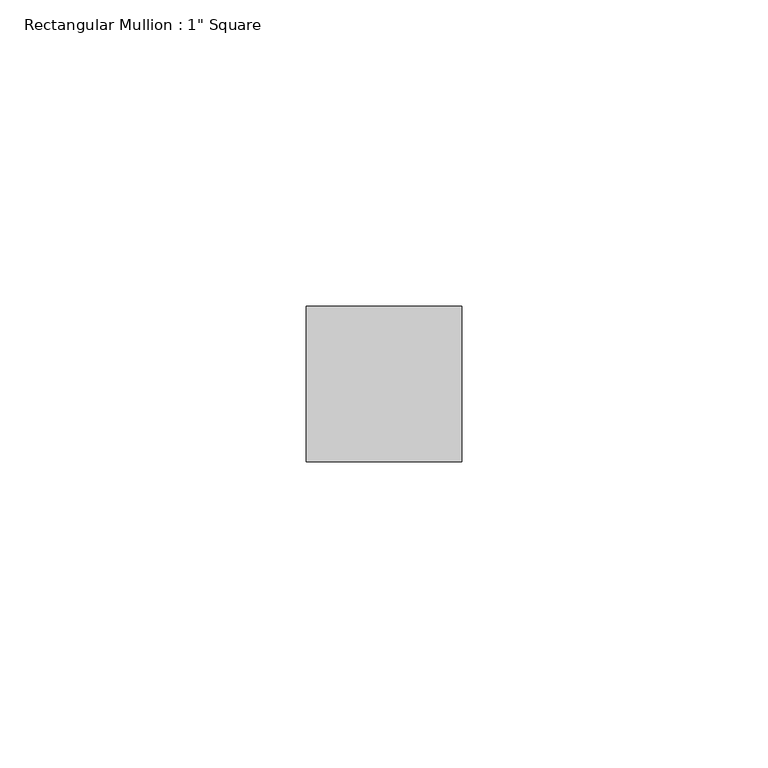
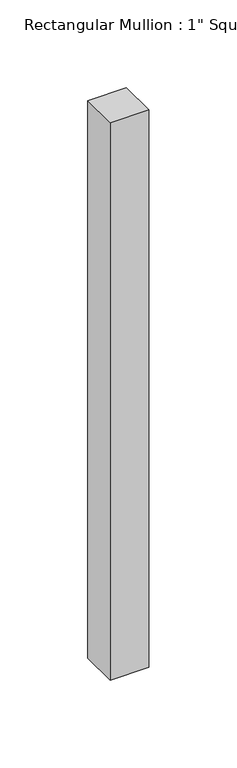
"""IFC4 building model written with IfcOpenShell, lengths in millimetres: member geometry."""

from ifc_helpers import new_model, si_unit, frame, origin, place, context, project, spatial, polyline, outline, extrude, source, transform, mapped, element, save


def member_66d82eec(model_context):
    return source(origin(), model_context, "Body", "SweptSolid", [
        extrude(outline(polyline([(12.7, 12.7), (12.7, -12.7), (-12.7, -12.7), (-12.7, 12.7), (12.7, 12.7)])), frame((0.0, 0.0, -387.35), z_axis=(0.0, 0.0, 1.0), x_axis=(1.0, 0.0, 0.0)), (0.0, 0.0, 1.0), 387.35),
    ])


if __name__ == "__main__":
    model = new_model("IFC4")
    model_context = context("Model", 3, world=origin())
    ifc_project = project(units=[si_unit("LENGTHUNIT", "METRE", prefix="MILLI")], contexts=[model_context])
    site = spatial("IfcSite", under=ifc_project)
    building = spatial("IfcBuilding", under=site)
    placement = place(None, origin())
    member_shape = member_66d82eec(model_context)
    element("IfcMember", 1, ObjectType="Rectangular Mullion : 1\" Square", at=placement, inside=building, context=model_context, shape_type="MappedRepresentation", body=[
        mapped(member_shape, transform((0.0, 0.0, 0.0), x_axis=(1.0, 0.0, 0.0), y_axis=(0.0, 1.0, 0.0), z_axis=(0.0, 0.0, 1.0))),
    ])
    save(model, "model.ifc")

# Revit data of these elements
# Type "Rectangular Mullion : 1\" Square"
#   built-in parameter 1007304 = 0.0833333 (stored number, unit not read)
#   built-in parameter 1007301 = 0.0416667 (stored number, unit not read)
#   built-in parameter 1007300 = 0.0416667 (stored number, unit not read)
# Element 1 (IfcMember, "Rectangular Mullion : 1\" Square")
#   Materials on its faces: "Aluminum"
# Materials
#   "Aluminum": class "Metal", colour RGB 247 247 247, transparency 0, Description = "Aluminum 6061", Cost = 0
